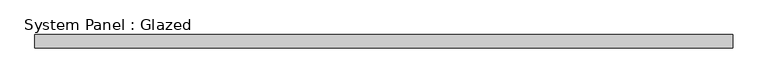
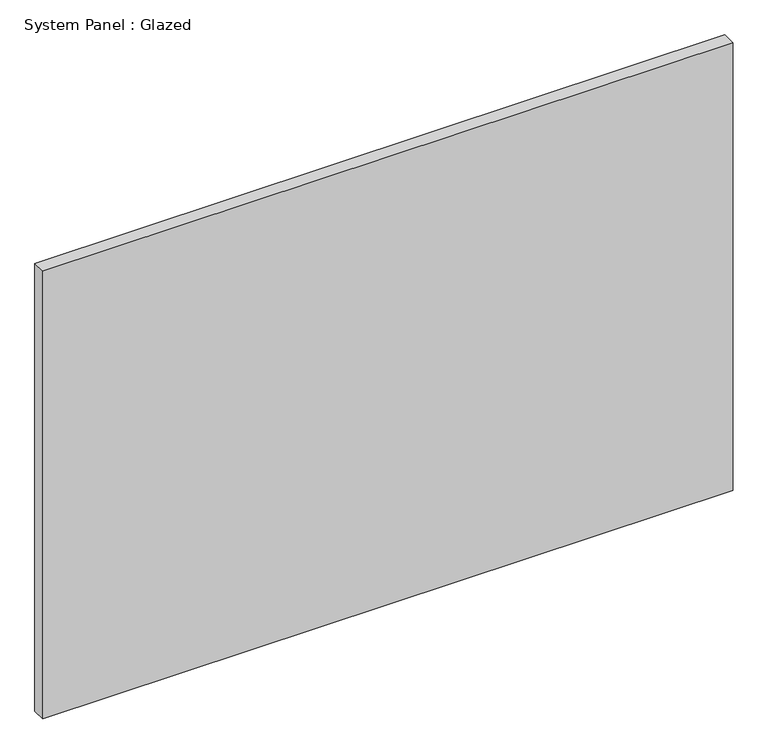
"""IFC4 building model written with IfcOpenShell, lengths in millimetres: plate geometry, System Panel : Glazed."""

from ifc_helpers import new_model, si_unit, origin, origin_with_axes, place, context, project, spatial, polyline, outline, extrude, source, transform, mapped, element, save


def system_panel_glazed_b56c0438(model_context):
    return source(origin(), model_context, "Body", "SweptSolid", [
        extrude(outline(polyline([(654.05, 19.05), (-654.05, 19.05), (-654.05, 44.45), (654.05, 44.45), (654.05, 19.05)])), origin_with_axes(), (0.0, 0.0, 1.0), 897.5064813),
    ])


if __name__ == "__main__":
    model = new_model("IFC4")
    model_context = context("Model", 3, world=origin())
    ifc_project = project(units=[si_unit("LENGTHUNIT", "METRE", prefix="MILLI")], contexts=[model_context])
    site = spatial("IfcSite", under=ifc_project)
    building = spatial("IfcBuilding", under=site)
    placement = place(None, origin())
    system_panel_glazed_shape = system_panel_glazed_b56c0438(model_context)
    element("IfcPlate", 1, ObjectType="System Panel : Glazed", at=placement, inside=building, context=model_context, shape_type="MappedRepresentation", body=[
        mapped(system_panel_glazed_shape, transform((0.0, 0.0, 0.0), x_axis=(1.0, 0.0, 0.0), y_axis=(0.0, 1.0, 0.0), z_axis=(0.0, 0.0, 1.0))),
    ])
    save(model, "model.ifc")

# Revit data of these elements
# Type "System Panel : Glazed"
#   Construction Type Id = "GSP4R"
#   Analytic Construction = "1/8 in Pilkington single glazing"
#   Visual Light Transmittance = 0.9
#   Solar Heat Gain Coefficient = 0.86
#   Heat Transfer Coefficient (U) = 1.18115 BTU/(h·ft²·°F)
#   Define Thermal Properties by = 1
# Element 1 (IfcPlate, "System Panel : Glazed")
#   Materials on its faces: "Glass"
# Materials
#   "Glass": class "Glass", colour RGB 0 128 192, transparency 0.75, Description = "Soda Lime Glass", Cost = 0
